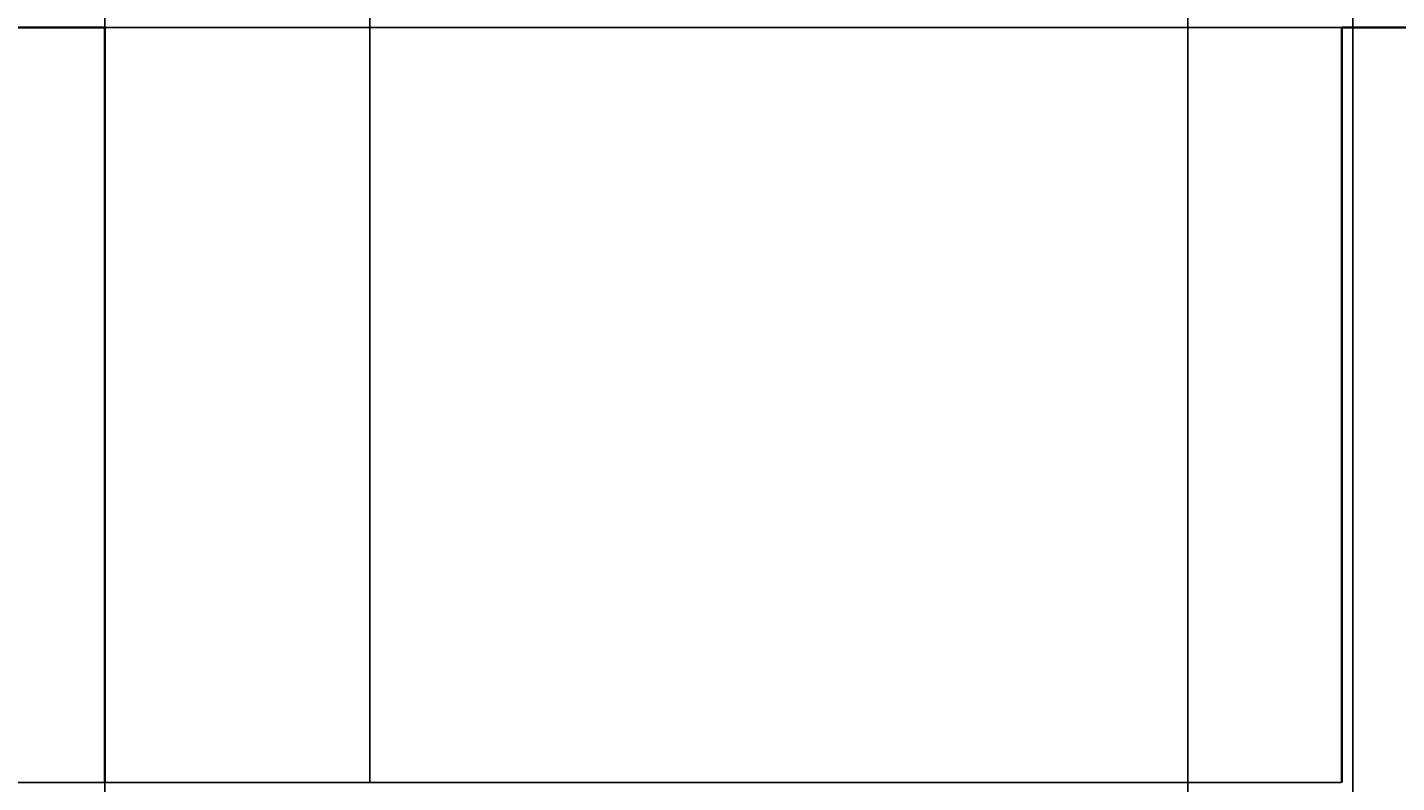
# Model space of a CAD drawing. Units: feet. Extents: x 100807 to 101423, y 154875 to 156331.
# Tile 6 of 8: x 101051 to 101176, y 156166 to 156235. Entities that reach past the tile are written whole.
import ezdxf

# ---------------------------------------------------------------- set-up
doc = ezdxf.new("R2010")
doc.units = ezdxf.units.FT
doc.layers.add('A-ANNO-DIMS', color=2, linetype='Continuous', lineweight=18)
doc.layers.add('A-WALL', color=7, linetype='Continuous', lineweight=35)
doc.styles.get("Standard").update_dxf_attribs({"font": 'arial.ttf'})
doc.dimstyles.get("Standard").update_dxf_attribs({"dimtxt": 0.18, "dimasz": 0.18, "dimexe": 0.18, "dimexo": 0.0625, "dimgap": 0.09, "dimtad": 0, "dimtih": 1, "dimtoh": 1, "dimdec": 4, "dimzin": 0, "dimdsep": 46, "dimtxsty": 'Standard', "dimcen": 0.09, "dimadec": 0, "dimazin": 0, "dimtfac": 1, "dimtdec": 4, "dimtofl": 0, "dimtmove": 0, "dimatfit": 3, "dimfxl": 1, "dimtolj": 1, "dimtzin": 0, "dimarcsym": 0})

# ---------------------------------------------------------------- blocks, each defined once
blk = doc.blocks.new('*D36')
at = {"layer": 'A-ANNO-DIMS', "color": 0, "lineweight": -2, "transparency": 16777216}
for p, q in [((101058.16, 155866.64), (101058.16, 156302.91)), ((101058.34, 156302.73), (101114.88, 156302.73)), ((101171.98, 156302.73), (101115.44, 156302.73)), ((101172.16, 155866.64), (101172.16, 156302.91))]:
    blk.add_line(p, q, dxfattribs=at)
at = {"layer": 'A-ANNO-DIMS', "color": 0, "transparency": 16777216}
for points in [[(101058.34, 156302.76), (101058.34, 156302.7), (101058.16, 156302.73)], [(101171.98, 156302.76), (101171.98, 156302.7), (101172.16, 156302.73)]]:
    blk.add_solid(points, dxfattribs=at)
at = {"layer": 'Defpoints', "color": 0, "transparency": 16777216}
for p in [(101172.16, 156302.73), (101058.16, 155866.58), (101172.16, 155866.58)]:
    blk.add_point(p, dxfattribs=at)
at = {"layer": 'A-ANNO-DIMS', "color": 0, "transparency": 16777216, "insert": (101115.16, 156302.73), "char_height": 0.18, "attachment_point": 5}
blk.add_mtext('\\A1;114', dxfattribs=at)
blk = doc.blocks.new('*D40')
at = {"layer": 'A-ANNO-DIMS', "color": 0, "lineweight": -2, "transparency": 16777216}
for p, q in [((101171.09, 156234.58), (100806.83, 156234.58)), ((100807.01, 156234.4), (100807.01, 156200.26)), ((100807.01, 156165.76), (100807.01, 156199.9)), ((101171.09, 156165.58), (100806.83, 156165.58))]:
    blk.add_line(p, q, dxfattribs=at)
at = {"layer": 'A-ANNO-DIMS', "color": 0, "transparency": 16777216}
for points in [[(100806.98, 156234.4), (100807.04, 156234.4), (100807.01, 156234.58)], [(100806.98, 156165.76), (100807.04, 156165.76), (100807.01, 156165.58)]]:
    blk.add_solid(points, dxfattribs=at)
at = {"layer": 'Defpoints', "color": 0, "transparency": 16777216}
for p in [(100807.01, 156234.58), (101171.16, 156234.58), (101171.16, 156165.58)]:
    blk.add_point(p, dxfattribs=at)
at = {"layer": 'A-ANNO-DIMS', "color": 0, "transparency": 16777216, "insert": (100807.01, 156200.08), "char_height": 0.18, "attachment_point": 5}
blk.add_mtext('\\A1;69', dxfattribs=at)
blk = doc.blocks.new('*D49')
at = {"layer": 'A-ANNO-DIMS', "color": 0, "lineweight": -2, "transparency": 16777216}
for p, q in [((101157.08, 155866.64), (101157.08, 156302.91)), ((101157.26, 156302.73), (101164.16, 156302.73)), ((101171.98, 156302.73), (101165.07, 156302.73)), ((101172.16, 155866.64), (101172.16, 156302.91))]:
    blk.add_line(p, q, dxfattribs=at)
at = {"layer": 'A-ANNO-DIMS', "color": 0, "transparency": 16777216}
for points in [[(101157.26, 156302.76), (101157.26, 156302.7), (101157.08, 156302.73)], [(101171.98, 156302.76), (101171.98, 156302.7), (101172.16, 156302.73)]]:
    blk.add_solid(points, dxfattribs=at)
at = {"layer": 'Defpoints', "color": 0, "transparency": 16777216}
for p in [(101172.16, 156302.73), (101157.08, 155866.58), (101172.16, 155866.58)]:
    blk.add_point(p, dxfattribs=at)
at = {"layer": 'A-ANNO-DIMS', "color": 0, "transparency": 16777216, "insert": (101164.62, 156302.73), "char_height": 0.18, "attachment_point": 5}
blk.add_mtext('\\A1;15.075', dxfattribs=at)
blk = doc.blocks.new('*D50')
at = {"layer": 'A-ANNO-DIMS', "color": 0, "lineweight": -2, "transparency": 16777216}
for p, q in [((101058.16, 156165.64), (101058.16, 156302.91)), ((101058.34, 156302.73), (101069.79, 156302.73)), ((101082.18, 156302.73), (101070.72, 156302.73)), ((101082.36, 156165.64), (101082.36, 156302.91))]:
    blk.add_line(p, q, dxfattribs=at)
at = {"layer": 'A-ANNO-DIMS', "color": 0, "transparency": 16777216}
for points in [[(101058.34, 156302.76), (101058.34, 156302.7), (101058.16, 156302.73)], [(101082.18, 156302.76), (101082.18, 156302.7), (101082.36, 156302.73)]]:
    blk.add_solid(points, dxfattribs=at)
at = {"layer": 'Defpoints', "color": 0, "transparency": 16777216}
for p in [(101082.36, 156302.73), (101058.16, 156165.58), (101082.36, 156165.58)]:
    blk.add_point(p, dxfattribs=at)
at = {"layer": 'A-ANNO-DIMS', "color": 0, "transparency": 16777216, "insert": (101070.26, 156302.73), "char_height": 0.18, "attachment_point": 5}
blk.add_mtext('\\A1;24.205', dxfattribs=at)

msp = doc.modelspace()

# ---------------------------------------------------------------- linework, layer by layer
at = {"layer": 'A-WALL'}
for p, q in [((100875.1564, 156234.5777), (101058.1564, 156234.5777)), ((101058.1564, 156234.5777), (101058.1564, 156210.5777)), ((101058.1564, 156234.5777), (101058.1564, 156222.5777)), ((101058.1564, 156234.5777), (101058.1564, 156210.5777)), ((101058.1564, 156234.5777), (101058.1564, 156165.5789)), ((101354.1564, 156234.5777), (101171.1564, 156234.5777)), ((101171.1564, 156234.5777), (101171.1564, 156210.5777)), ((101171.1564, 156234.5777), (101171.1564, 156222.5777)), ((101171.1564, 156234.5777), (101171.1564, 156165.5789))]:
    msp.add_line(p, q, dxfattribs=at)

# ---------------------------------------------------------------- dimensions: what is measured, and where the dimension line sits
at = {"layer": 'A-ANNO-DIMS'}
for base, p1, p2, override, picture, middle in [((101172.1564, 156302.7277), (101058.1564, 155866.5789), (101172.1564, 155866.5789), {"dimdec": 0, "dimlfac": 1, "dimrnd": 0, "dimzin": 0, "dimdsep": 46, "dimlunit": 2}, '*D36', (101115.1564, 156302.7277)), ((101082.3615, 156302.7277), (101058.1564, 156165.5789), (101082.3615, 156165.5789), {"dimdec": 3, "dimlfac": 1, "dimrnd": 0, "dimzin": 0, "dimdsep": 46, "dimlunit": 2}, '*D50', (101070.259, 156302.7277)), ((101172.1564, 156302.7277), (101157.0816, 155866.5789), (101172.1564, 155866.5789), {"dimdec": 3, "dimlfac": 1, "dimrnd": 0, "dimzin": 0, "dimdsep": 46, "dimlunit": 2}, '*D49', (101164.619, 156302.7277))]:
    dim = msp.add_linear_dim(base=base, p1=p1, p2=p2, dimstyle='Standard', override=override, dxfattribs=at)
    dim.commit()
    dim.dimension.update_dxf_attribs({"geometry": picture, "text_midpoint": middle})
dim = msp.add_linear_dim(base=(100807.0064, 156234.5777), p1=(101171.1564, 156165.5789), p2=(101171.1564, 156234.5777), angle=90, dimstyle='Standard', override={"dimdec": 0, "dimlfac": 1, "dimrnd": 0, "dimzin": 0, "dimdsep": 46, "dimlunit": 2}, dxfattribs=at)
dim.commit()
dim.dimension.update_dxf_attribs({"geometry": '*D40', "text_midpoint": (100807.0064, 156200.0783)})

doc.saveas('drawing.dxf')
